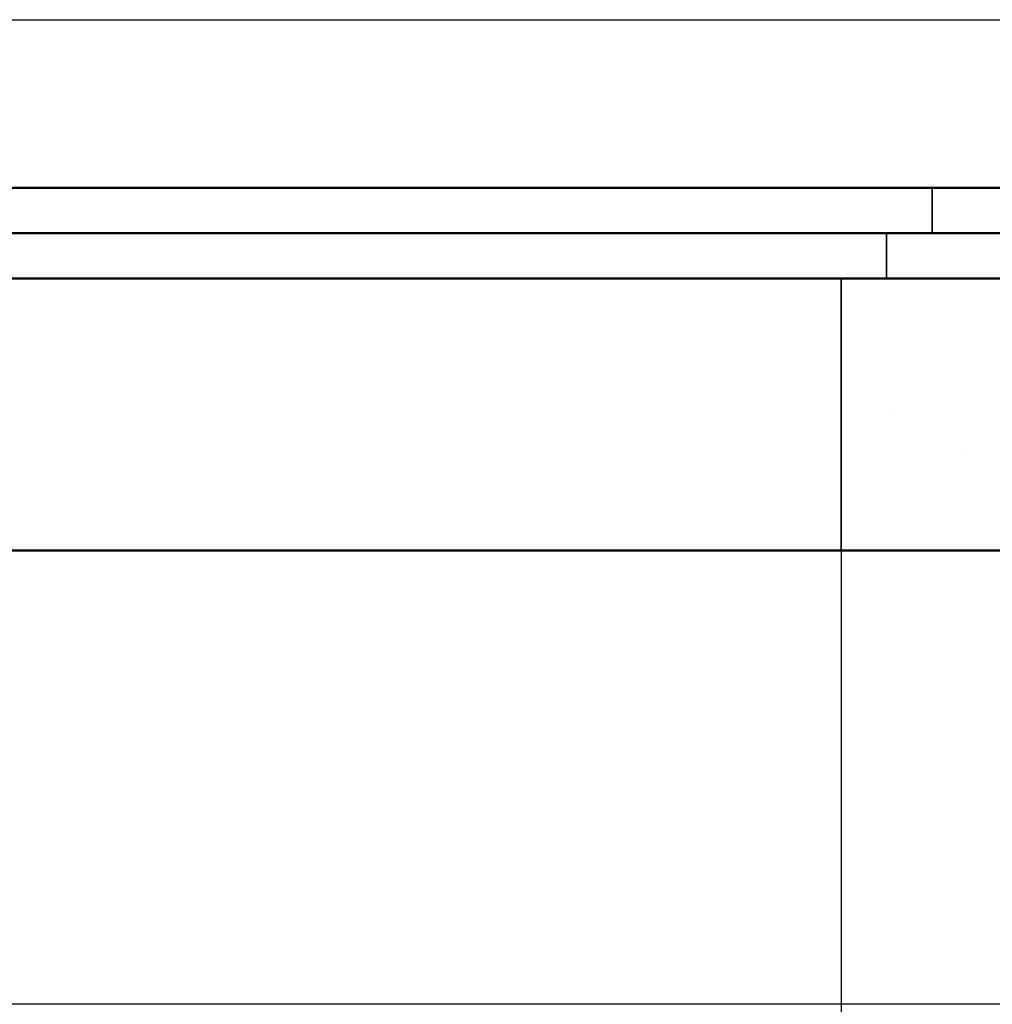
# Model space of a CAD drawing. Units: inches. Extents: x 2812 to 3051, y 1398 to 1659.
# Tile 26 of 65: x 2923 to 2945, y 1472 to 1494. Entities that reach past the tile are written whole.
import ezdxf

# ---------------------------------------------------------------- set-up
doc = ezdxf.new("R2010")
doc.units = ezdxf.units.IN
for name, color, linetype, lineweight in [('A-ANNO-DIMS', 2, 'Continuous', 18), ('S-CONC', 7, 'Continuous', 50), ('S-CONC-PATT', 8, 'Continuous', 18), ('S-CONC-SLAB', 7, 'Continuous', 35)]:
    doc.layers.add(name, color=color, linetype=linetype, lineweight=lineweight)
doc.styles.get("Standard").update_dxf_attribs({"font": 'arial.ttf'})
doc.dimstyles.get("Standard").update_dxf_attribs({"dimtxt": 0.18, "dimasz": 0.18, "dimexe": 0.18, "dimexo": 0.0625, "dimgap": 0.09, "dimtad": 0, "dimtih": 1, "dimtoh": 1, "dimdec": 4, "dimzin": 0, "dimdsep": 46, "dimtxsty": 'Standard', "dimcen": 0.09, "dimadec": 0, "dimazin": 0, "dimtfac": 1, "dimtdec": 4, "dimtofl": 0, "dimtmove": 0, "dimatfit": 3, "dimfxl": 1, "dimtolj": 1, "dimtzin": 0, "dimarcsym": 0})

# ---------------------------------------------------------------- blocks, each defined once
blk = doc.blocks.new('COVER-SLAB-PLAN')
for p, q in [((2, 7), (2, 8)), ((1, 6), (1, 7)), ((1, 7), (2, 7)), ((0, 6), (0, 0)), ((0, 6), (1, 6))]:
    blk.add_line(p, q)
blk = doc.blocks.new('*D45')
at = {"layer": 'A-ANNO-DIMS', "color": 0, "lineweight": -2, "transparency": 16777216}
for p, q in [((2896.385, 1487.973), (2896.385, 1397.505)), ((2941.385, 1487.973), (2941.385, 1397.505)), ((2896.565, 1397.685), (2918.662, 1397.685)), ((2941.205, 1397.685), (2919.108, 1397.685))]:
    blk.add_line(p, q, dxfattribs=at)
at = {"layer": 'A-ANNO-DIMS', "color": 0, "transparency": 16777216}
for points in [[(2896.565, 1397.715), (2896.565, 1397.655), (2896.385, 1397.685)], [(2941.205, 1397.715), (2941.205, 1397.655), (2941.385, 1397.685)]]:
    blk.add_solid(points, dxfattribs=at)
at = {"layer": 'Defpoints', "color": 0, "transparency": 16777216}
for p in [(2896.385, 1488.035), (2941.385, 1488.035), (2941.385, 1397.685)]:
    blk.add_point(p, dxfattribs=at)
at = {"layer": 'A-ANNO-DIMS', "color": 0, "transparency": 16777216, "insert": (2918.885, 1397.685), "char_height": 0.18, "attachment_point": 5}
blk.add_mtext('\\A1;45', dxfattribs=at)
blk = doc.blocks.new('*D46')
at = {"layer": 'A-ANNO-DIMS', "color": 0, "lineweight": -2, "transparency": 16777216}
for p, q in [((2941.385, 1487.973), (2941.385, 1397.505)), ((2970.385, 1487.973), (2970.385, 1397.505)), ((2941.565, 1397.685), (2955.664, 1397.685)), ((2970.205, 1397.685), (2956.106, 1397.685))]:
    blk.add_line(p, q, dxfattribs=at)
at = {"layer": 'A-ANNO-DIMS', "color": 0, "transparency": 16777216}
for points in [[(2941.565, 1397.715), (2941.565, 1397.655), (2941.385, 1397.685)], [(2970.205, 1397.715), (2970.205, 1397.655), (2970.385, 1397.685)]]:
    blk.add_solid(points, dxfattribs=at)
at = {"layer": 'Defpoints', "color": 0, "transparency": 16777216}
for p in [(2941.385, 1488.035), (2970.385, 1488.035), (2970.385, 1397.685)]:
    blk.add_point(p, dxfattribs=at)
at = {"layer": 'A-ANNO-DIMS', "color": 0, "transparency": 16777216, "insert": (2955.885, 1397.685), "char_height": 0.18, "attachment_point": 5}
blk.add_mtext('\\A1;29', dxfattribs=at)
blk = doc.blocks.new('*D55')
at = {"layer": 'A-ANNO-DIMS', "color": 0, "lineweight": -2, "transparency": 16777216}
for p, q in [((2850.811, 1493.738), (3051.178, 1493.738)), ((3050.998, 1493.558), (3050.998, 1491.069)), ((3050.998, 1488.215), (3050.998, 1490.705)), ((2850.811, 1488.035), (3051.178, 1488.035))]:
    blk.add_line(p, q, dxfattribs=at)
at = {"layer": 'A-ANNO-DIMS', "color": 0, "transparency": 16777216}
for points in [[(3050.968, 1493.558), (3051.028, 1493.558), (3050.998, 1493.738)], [(3050.968, 1488.215), (3051.028, 1488.215), (3050.998, 1488.035)]]:
    blk.add_solid(points, dxfattribs=at)
at = {"layer": 'Defpoints', "color": 0, "transparency": 16777216}
for p in [(2850.748, 1493.738), (3050.998, 1493.738), (2850.748, 1488.035)]:
    blk.add_point(p, dxfattribs=at)
at = {"layer": 'A-ANNO-DIMS', "color": 0, "transparency": 16777216, "insert": (3050.998, 1490.887), "char_height": 0.18, "attachment_point": 5}
blk.add_mtext('\\A1;5.703', dxfattribs=at)
blk = doc.blocks.new('*D77')
at = {"layer": 'A-ANNO-DIMS', "color": 0, "lineweight": -2, "transparency": 16777216}
for p, q in [((2961.322, 1472.035), (2811.806, 1472.035)), ((2811.986, 1471.855), (2811.986, 1461.436)), ((2811.986, 1450.654), (2811.986, 1461.073)), ((2963.812, 1450.474), (2811.806, 1450.474))]:
    blk.add_line(p, q, dxfattribs=at)
at = {"layer": 'A-ANNO-DIMS', "color": 0, "transparency": 16777216}
for points in [[(2811.956, 1471.855), (2812.016, 1471.855), (2811.986, 1472.035)], [(2811.956, 1450.654), (2812.016, 1450.654), (2811.986, 1450.474)]]:
    blk.add_solid(points, dxfattribs=at)
at = {"layer": 'Defpoints', "color": 0, "transparency": 16777216}
for p in [(2811.986, 1472.035), (2961.385, 1472.035), (2963.874, 1450.474)]:
    blk.add_point(p, dxfattribs=at)
at = {"layer": 'A-ANNO-DIMS', "color": 0, "transparency": 16777216, "insert": (2811.986, 1461.255), "char_height": 0.18, "attachment_point": 5}
blk.add_mtext('\\A1;21.56', dxfattribs=at)

msp = doc.modelspace()

# ---------------------------------------------------------------- hatches: boundary and pattern name
at = {"layer": 'S-CONC-PATT'}
h = msp.add_hatch(dxfattribs=at)
h.set_pattern_fill('AR-SAND', color=256, scale=0.3)
h.paths.add_polyline_path([(3036.3849, 1416.0354), (3027.3849, 1416.0354), (2826.3849, 1416.0354), (2826.3849, 1410.0354), (2835.3849, 1410.0354), (3036.3849, 1410.0354)])
h.paths.add_polyline_path([(2970.3849, 1488.0354), (2969.3849, 1488.0354), (2941.3849, 1488.0354), (2941.3849, 1482.0354), (2970.3849, 1482.0354)])
h.paths.add_polyline_path([(3036.3849, 1488.0354), (3035.3849, 1488.0354), (3006.3849, 1488.0354), (3006.3849, 1482.0354), (3027.3849, 1482.0354), (3036.3849, 1482.0354)])
h.paths.add_polyline_path([(3034.3849, 1490.0354), (3008.3849, 1490.0354), (3008.3849, 1489.0354), (3034.3849, 1489.0354)])
h.paths.add_polyline_path([(3035.3849, 1489.0354), (3034.3849, 1489.0354), (3007.3849, 1489.0354), (3007.3849, 1488.0354), (3035.3849, 1488.0354)])
h.paths.add_polyline_path([(2968.3849, 1490.0354), (2943.3849, 1490.0354), (2943.3849, 1489.0354), (2968.3849, 1489.0354)])
h.paths.add_polyline_path([(2969.3849, 1489.0354), (2968.3849, 1489.0354), (2942.3849, 1489.0354), (2942.3849, 1488.0354), (2969.3849, 1488.0354)])
h.paths.add_polyline_path([(2896.3849, 1488.0354), (2826.3849, 1488.0354), (2826.3849, 1482.0354), (2896.3849, 1482.0354)])
h.paths.add_polyline_path([(2895.3849, 1489.0354), (2894.3849, 1489.0354), (2827.3849, 1489.0354), (2827.3849, 1488.0354), (2895.3849, 1488.0354)])
h.paths.add_polyline_path([(2894.3849, 1490.0354), (2828.3849, 1490.0354), (2828.3849, 1489.0354), (2894.3849, 1489.0354)])
h = msp.add_hatch(dxfattribs=at)
h.set_pattern_fill('AR-CONC', color=256, scale=0.3)
h.paths.add_polyline_path([(2896.3849, 1488.0354), (2826.3849, 1488.0354), (2826.3849, 1482.0354), (2896.3849, 1482.0354)])
h.paths.add_polyline_path([(2970.3849, 1488.0354), (2941.3849, 1488.0354), (2941.3849, 1482.0354), (2970.3849, 1482.0354)])
h.paths.add_polyline_path([(2968.3849, 1490.0354), (2943.3849, 1490.0354), (2943.3849, 1489.0354), (2968.3849, 1489.0354)])
h.paths.add_polyline_path([(2969.3849, 1489.0354), (2968.3849, 1489.0354), (2943.3849, 1489.0354), (2942.3849, 1489.0354), (2942.3849, 1488.0354), (2969.3849, 1488.0354)])
h.paths.add_polyline_path([(3036.3849, 1488.0354), (3035.3849, 1488.0354), (3006.3849, 1488.0354), (3006.3849, 1482.0354), (3027.3849, 1482.0354), (3036.3849, 1482.0354)])
h.paths.add_polyline_path([(3035.3849, 1489.0354), (3034.3849, 1489.0354), (3007.3849, 1489.0354), (3007.3849, 1488.0354), (3035.3849, 1488.0354)])
h.paths.add_polyline_path([(3034.3849, 1490.0354), (3008.3849, 1490.0354), (3008.3849, 1489.0354), (3034.3849, 1489.0354)])
h.paths.add_polyline_path([(2895.3849, 1489.0354), (2894.3849, 1489.0354), (2827.3849, 1489.0354), (2827.3849, 1488.0354), (2895.3849, 1488.0354)])
h.paths.add_polyline_path([(2894.3849, 1490.0354), (2828.3849, 1490.0354), (2828.3849, 1489.0354), (2894.3849, 1489.0354)])

# ---------------------------------------------------------------- linework, layer by layer
at = {"layer": 'S-CONC'}
for p, q in [((3034.3849, 1490.0354), (2850.7485, 1490.0354)), ((2850.7485, 1489.0354), (3035.3849, 1489.0354)), ((2850.7485, 1488.0354), (3036.3849, 1488.0354)), ((2850.7485, 1482.0354), (3027.3849, 1482.0354))]:
    msp.add_line(p, q, dxfattribs=at)

# ---------------------------------------------------------------- block references
at = {"layer": 'S-CONC-SLAB'}
msp.add_blockref('COVER-SLAB-PLAN', (2941.385, 1482.035), dxfattribs=at)

# ---------------------------------------------------------------- dimensions: what is measured, and where the dimension line sits
at = {"layer": 'A-ANNO-DIMS'}
for base, p1, p2, override, picture, middle in [((3050.998, 1493.7383), (2850.7485, 1488.0354), (2850.7485, 1493.7383), {"dimdec": 3, "dimlfac": 1, "dimrnd": 0, "dimzin": 0, "dimdsep": 46, "dimlunit": 2}, '*D55', (3050.998, 1490.8868)), ((2811.9855, 1472.0354), (2963.8741, 1450.4738), (2961.3849, 1472.0354), {"dimdec": 2, "dimlfac": 1, "dimrnd": 0, "dimzin": 0, "dimdsep": 46, "dimlunit": 2}, '*D77', (2811.9855, 1461.2546))]:
    dim = msp.add_linear_dim(base=base, p1=p1, p2=p2, angle=90, dimstyle='Standard', override=override, dxfattribs=at)
    dim.commit()
    dim.dimension.update_dxf_attribs({"geometry": picture, "text_midpoint": middle})
for base, p1, p2, picture, middle in [((2941.3849, 1397.6854), (2896.3849, 1488.0354), (2941.3849, 1488.0354), '*D45', (2918.8849, 1397.6854)), ((2970.3849, 1397.6854), (2941.3849, 1488.0354), (2970.3849, 1488.0354), '*D46', (2955.8849, 1397.6854))]:
    dim = msp.add_linear_dim(base=base, p1=p1, p2=p2, dimstyle='Standard', override={"dimdec": 0, "dimlfac": 1, "dimrnd": 0, "dimzin": 0, "dimdsep": 46, "dimlunit": 2}, dxfattribs=at)
    dim.commit()
    dim.dimension.update_dxf_attribs({"geometry": picture, "text_midpoint": middle})

doc.saveas('drawing.dxf')
